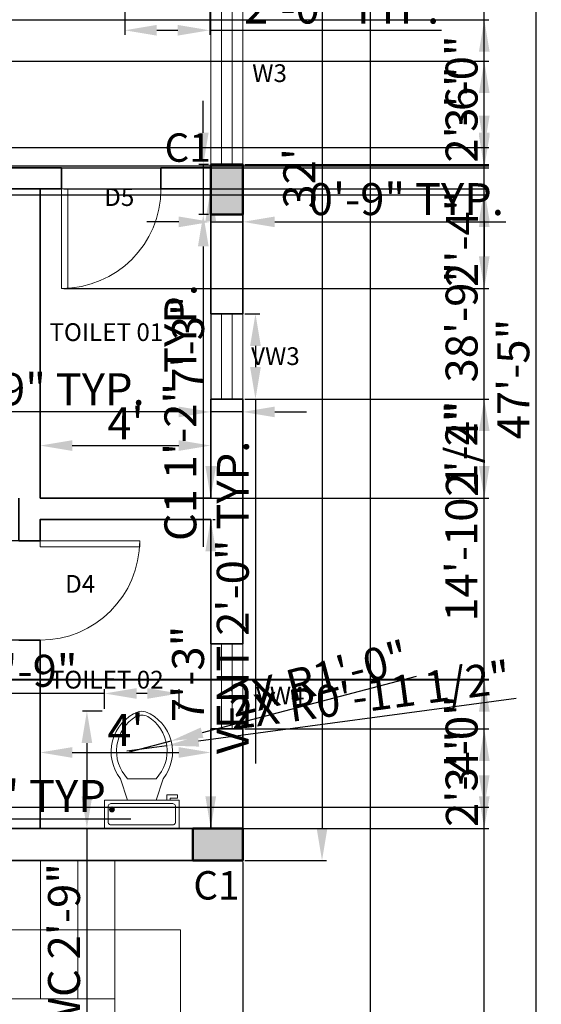
# Model space of a CAD drawing. Units: inches. Extents: x 2621 to 6190, y 513 to 1320.
# Tile 9 of 11: x 3160 to 3306, y 661 to 939. Entities that reach past the tile are written whole.
import ezdxf

# ---------------------------------------------------------------- set-up
doc = ezdxf.new("R2010")
doc.units = ezdxf.units.IN
for name, color, linetype, lineweight in [('A-ANNO-DIMS', 5, 'Continuous', 18), ('A-ANNO-TEXT', 7, 'Continuous', 18), ('A-AREA-IDEN', 7, 'Continuous', 25), ('A-FLOR-CASE', 30, 'Continuous', 18), ('A-FLOR-FIXT', 30, 'Continuous', 18), ('A-WALL', 7, 'Continuous', 35), ('C-PROP', 7, 'Continuous', 25), ('columns', 2, 'Continuous', 50), ('door', 1, 'Continuous', 18), ('S-COLS-IDEN', 2, 'Continuous', 25), ('S-COLS-PATT', 2, 'Continuous', 13), ('stairs', 104, 'Continuous', 18), ('window', 172, 'Continuous', 18)]:
    doc.layers.add(name, color=color, linetype=linetype, lineweight=lineweight)
doc.styles.get("Standard").update_dxf_attribs({"font": 'arial.ttf'})
doc.dimstyles.new('ISO-25', dxfattribs={"dimtxt": 9, "dimasz": 9, "dimexe": 1.25, "dimexo": 0.625, "dimtad": 1, "dimlunit": 3, "dimtxsty": 'Standard', "dimcen": 2.5, "dimadec": 0, "dimazin": 0, "dimtfac": 1, "dimtmove": 0, "dimatfit": 3, "dimfxl": 1, "dimarcsym": 0})

# ---------------------------------------------------------------- blocks, each defined once
blk = doc.blocks.new('*U4')
for p, q in [((0, 0), (0, 6)), ((28, 0), (28, 6))]:
    blk.add_line(p, q)
blk.add_lwpolyline([(0, 0), (0, -28), (1.75, -28), (1.75, 0)], close=True)
blk.add_arc((0, 0), 28, 270, 0)
blk = doc.blocks.new('*U3')
for p, q in [((-28, 0), (-28, 6)), ((0, 0), (0, 6))]:
    blk.add_line(p, q)
blk.add_lwpolyline([(0, 0), (0, -28), (-1.75, -28), (-1.75, 0)], close=True)
blk.add_arc((0, 0), 28, 180, 270)
blk = doc.blocks.new('Toilet - top')
for p, q in [((9.5, -6), (9.5, -2)), ((-8, -8.5), (-8, -8)), ((-7, -8), (-7, -9.5)), ((-4, -8), (-6, -14)), ((4, -8), (6, -14)), ((-10, -8.5), (-8, -8.5)), ((-10, -9.5), (-10, -8.5)), ((-7, -9.5), (-10, -9.5)), ((4, -14), (-4, -14))]:
    blk.add_line(p, q)
blk.add_lwpolyline([(10.5, -8), (10.5, 0), (-10.5, 0), (-10.5, -8)], close=True)
for points in [[(-9.5, -2), (-9.5, -6)], [(8.5, -1), (-8.5, -1)], [(-8.5, -7), (8.5, -7)]]:
    blk.add_lwpolyline(points)
for centre, radius, start, end in [((-8.62, -1.88), 0.884, 81.8699, 188.1301), ((8.62, -1.88), 0.884, 351.8699, 98.1301), ((-8.62, -6.12), 0.884, 171.8699, 278.1301), ((8.62, -6.12), 0.884, 261.8699, 8.1301), ((3.52, -21.58), 12.17, 141.4691, 247.9714), ((4.2, -21.82), 11.33, 136.3677, 238.9468), ((-3.52, -21.58), 12.17, 292.0284, 38.5307), ((-4.2, -21.82), 11.33, 301.053, 43.6321), ((0, -27.88), 4, 245.7318, 294.2682), ((0, -29), 4, 254.8605, 285.1395)]:
    blk.add_arc(centre, radius, start, end)
blk = doc.blocks.new('*D29')
at = {"layer": 'A-ANNO-DIMS', "color": 0, "lineweight": -2, "transparency": 16777216}
for p, q in [((3214.01, 797.89), (3214.63, 797.89)), ((3213.38, 788.89), (3213.38, 719.89)), ((3214.01, 710.89), (3214.63, 710.89))]:
    blk.add_line(p, q, dxfattribs=at)
at = {"layer": 'A-ANNO-DIMS', "color": 0, "transparency": 16777216}
for points in [[(3211.88, 788.89), (3214.88, 788.89), (3213.38, 797.89)], [(3211.88, 719.89), (3214.88, 719.89), (3213.38, 710.89)]]:
    blk.add_solid(points, dxfattribs=at)
at = {"layer": 'Defpoints', "color": 0, "transparency": 16777216}
for p in [(3213.38, 797.89), (3213.38, 710.89), (3213.38, 710.89)]:
    blk.add_point(p, dxfattribs=at)
at = {"layer": 'A-ANNO-DIMS', "color": 0, "transparency": 16777216, "insert": (3208.16, 754.39), "char_height": 9, "attachment_point": 5, "rotation": 90}
blk.add_mtext('7\'-3"', dxfattribs=at)
blk = doc.blocks.new('*D30')
at = {"layer": 'A-ANNO-DIMS', "color": 0, "lineweight": -2, "transparency": 16777216}
for p, q in [((3165.38, 729.52), (3165.38, 733.53)), ((3174.38, 732.28), (3204.38, 732.28)), ((3213.38, 731.63), (3213.38, 733.53))]:
    blk.add_line(p, q, dxfattribs=at)
at = {"layer": 'A-ANNO-DIMS', "color": 0, "transparency": 16777216}
for points in [[(3174.38, 733.78), (3174.38, 730.78), (3165.38, 732.28)], [(3204.38, 733.78), (3204.38, 730.78), (3213.38, 732.28)]]:
    blk.add_solid(points, dxfattribs=at)
at = {"layer": 'Defpoints', "color": 0, "transparency": 16777216}
for p in [(3213.38, 732.28), (3213.38, 731.01), (3165.38, 728.89)]:
    blk.add_point(p, dxfattribs=at)
at = {"layer": 'A-ANNO-DIMS', "color": 0, "transparency": 16777216, "insert": (3189.38, 737.4), "char_height": 9, "attachment_point": 5}
blk.add_mtext("4'", dxfattribs=at)
blk = doc.blocks.new('*D31')
at = {"layer": 'A-ANNO-DIMS', "color": 0, "lineweight": -2, "transparency": 16777216}
for p, q in [((3165.38, 819.75), (3165.38, 817.42)), ((3174.38, 818.67), (3204.38, 818.67)), ((3213.38, 819.75), (3213.38, 817.42))]:
    blk.add_line(p, q, dxfattribs=at)
at = {"layer": 'A-ANNO-DIMS', "color": 0, "transparency": 16777216}
for points in [[(3174.38, 820.17), (3174.38, 817.17), (3165.38, 818.67)], [(3204.38, 820.17), (3204.38, 817.17), (3213.38, 818.67)]]:
    blk.add_solid(points, dxfattribs=at)
at = {"layer": 'Defpoints', "color": 0, "transparency": 16777216}
for p in [(3165.38, 820.37), (3213.38, 820.37), (3213.38, 818.67)]:
    blk.add_point(p, dxfattribs=at)
at = {"layer": 'A-ANNO-DIMS', "color": 0, "transparency": 16777216, "insert": (3189.38, 823.79), "char_height": 9, "attachment_point": 5}
blk.add_mtext("4'", dxfattribs=at)
blk = doc.blocks.new('*D32')
at = {"layer": 'A-ANNO-DIMS', "color": 0, "lineweight": -2, "transparency": 16777216}
for p, q in [((3207.01, 890.89), (3214.63, 890.89)), ((3213.38, 881.89), (3213.38, 812.89)), ((3207.01, 803.89), (3214.63, 803.89))]:
    blk.add_line(p, q, dxfattribs=at)
at = {"layer": 'A-ANNO-DIMS', "color": 0, "transparency": 16777216}
for points in [[(3211.88, 881.89), (3214.88, 881.89), (3213.38, 890.89)], [(3211.88, 812.89), (3214.88, 812.89), (3213.38, 803.89)]]:
    blk.add_solid(points, dxfattribs=at)
at = {"layer": 'Defpoints', "color": 0, "transparency": 16777216}
for p in [(3206.38, 890.89), (3206.38, 803.89), (3213.38, 803.89)]:
    blk.add_point(p, dxfattribs=at)
at = {"layer": 'A-ANNO-DIMS', "color": 0, "transparency": 16777216, "insert": (3208.16, 847.39), "char_height": 9, "attachment_point": 5, "rotation": 90}
blk.add_mtext('7\'-3"', dxfattribs=at)
blk = doc.blocks.new('*D35')
at = {"layer": 'A-ANNO-DIMS', "color": 0, "lineweight": -2, "transparency": 16777216}
for p, q in [((3223.01, 1085.89), (3245.96, 1085.89)), ((3244.71, 1076.89), (3244.71, 710.89)), ((3223.01, 701.89), (3245.96, 701.89))]:
    blk.add_line(p, q, dxfattribs=at)
at = {"layer": 'A-ANNO-DIMS', "color": 0, "transparency": 16777216}
for points in [[(3243.21, 1076.89), (3246.21, 1076.89), (3244.71, 1085.89)], [(3243.21, 710.89), (3246.21, 710.89), (3244.71, 701.89)]]:
    blk.add_solid(points, dxfattribs=at)
at = {"layer": 'Defpoints', "color": 0, "transparency": 16777216}
for p in [(3222.38, 1085.89), (3222.38, 701.89), (3244.71, 701.89)]:
    blk.add_point(p, dxfattribs=at)
at = {"layer": 'A-ANNO-DIMS', "color": 0, "transparency": 16777216, "insert": (3239.48, 893.89), "char_height": 9, "attachment_point": 5, "rotation": 90}
blk.add_mtext("32'", dxfattribs=at)
blk = doc.blocks.new('*D39')
at = {"layer": 'A-ANNO-DIMS', "color": 0, "lineweight": -2, "transparency": 16777216}
for p, q in [((3259.01, 1121.89), (3306.19, 1121.89)), ((3304.94, 1112.89), (3304.94, 561.89)), ((3259.01, 552.89), (3306.19, 552.89))]:
    blk.add_line(p, q, dxfattribs=at)
at = {"layer": 'A-ANNO-DIMS', "color": 0, "transparency": 16777216}
for points in [[(3303.44, 1112.89), (3306.44, 1112.89), (3304.94, 1121.89)], [(3303.44, 561.89), (3306.44, 561.89), (3304.94, 552.89)]]:
    blk.add_solid(points, dxfattribs=at)
at = {"layer": 'Defpoints', "color": 0, "transparency": 16777216}
for p in [(3258.38, 1121.89), (3258.38, 552.89), (3304.94, 552.89)]:
    blk.add_point(p, dxfattribs=at)
at = {"layer": 'A-ANNO-DIMS', "color": 0, "transparency": 16777216, "insert": (3299.73, 837.39), "char_height": 9, "attachment_point": 5, "rotation": 90}
blk.add_mtext('47\'-5"', dxfattribs=at)
blk = doc.blocks.new('WIN-VENT-24IN')
for p, q in [((9, 24), (0, 24)), ((0, 24), (0, 0)), ((3, 24), (3, 0)), ((6, 24), (6, 0)), ((9, 0), (9, 24)), ((0, 0), (9, 0))]:
    blk.add_line(p, q)
blk = doc.blocks.new('WIN-48IN')
for p, q in [((48, 9), (0, 9)), ((0, 9), (0, 0)), ((48, 0), (48, 9)), ((0, 6), (48, 6)), ((0, 3), (48, 3)), ((0, 0), (48, 0))]:
    blk.add_line(p, q)
blk = doc.blocks.new('COL-C1-9X14')
blk.add_lwpolyline([(0, 0), (0, 9), (14, 9), (14, 0)], close=True)
blk = doc.blocks.new('*D51')
at = {"layer": 'A-ANNO-DIMS', "color": 0, "lineweight": -2, "transparency": 16777216}
for p, q in [((3211.28, 906.74), (3211.28, 915.74)), ((3212.76, 897.74), (3210.03, 897.74)), ((3211.28, 897.74), (3211.28, 883.74)), ((3212.76, 883.74), (3210.03, 883.74)), ((3211.28, 874.74), (3211.28, 790.17))]:
    blk.add_line(p, q, dxfattribs=at)
at = {"layer": 'A-ANNO-DIMS', "color": 0, "transparency": 16777216}
for points in [[(3209.78, 906.74), (3212.78, 906.74), (3211.28, 897.74)], [(3209.78, 874.74), (3212.78, 874.74), (3211.28, 883.74)]]:
    blk.add_solid(points, dxfattribs=at)
at = {"layer": 'Defpoints', "color": 0, "transparency": 16777216}
for p in [(3213.38, 897.74), (3211.28, 883.74), (3213.38, 883.74)]:
    blk.add_point(p, dxfattribs=at)
at = {"layer": 'A-ANNO-DIMS', "color": 0, "transparency": 16777216, "insert": (3206, 827.96), "char_height": 9, "attachment_point": 5, "rotation": 90}
blk.add_mtext('C1 1\'-2" TYP.', dxfattribs=at)
blk = doc.blocks.new('*D52')
at = {"layer": 'A-ANNO-DIMS', "color": 0, "lineweight": -2, "transparency": 16777216}
for p, q in [((3204.38, 881.64), (3195.38, 881.64)), ((3213.38, 883.12), (3213.38, 880.39)), ((3213.38, 881.64), (3222.38, 881.64)), ((3222.38, 883.12), (3222.38, 880.39)), ((3231.38, 881.64), (3296.49, 881.64))]:
    blk.add_line(p, q, dxfattribs=at)
at = {"layer": 'A-ANNO-DIMS', "color": 0, "transparency": 16777216}
for points in [[(3204.38, 883.14), (3204.38, 880.14), (3213.38, 881.64)], [(3231.38, 883.14), (3231.38, 880.14), (3222.38, 881.64)]]:
    blk.add_solid(points, dxfattribs=at)
at = {"layer": 'Defpoints', "color": 0, "transparency": 16777216}
for p in [(3213.38, 883.74), (3222.38, 883.74), (3222.38, 881.64)]:
    blk.add_point(p, dxfattribs=at)
at = {"layer": 'A-ANNO-DIMS', "color": 0, "transparency": 16777216, "insert": (3268.44, 886.87), "char_height": 9, "attachment_point": 5}
blk.add_mtext('0\'-9" TYP.', dxfattribs=at)
blk = doc.blocks.new('*D53')
at = {"layer": 'A-ANNO-DIMS', "color": 0, "lineweight": -2, "transparency": 16777216}
for p, q in [((3012.32, 713.59), (3003.32, 713.59)), ((3021.32, 711.51), (3021.32, 714.84)), ((3021.32, 713.59), (3039.32, 713.59)), ((3039.32, 711.51), (3039.32, 714.84)), ((3048.32, 713.59), (3190.87, 713.59))]:
    blk.add_line(p, q, dxfattribs=at)
at = {"layer": 'A-ANNO-DIMS', "color": 0, "transparency": 16777216}
for points in [[(3012.32, 715.09), (3012.32, 712.09), (3021.32, 713.59)], [(3048.32, 715.09), (3048.32, 712.09), (3039.32, 713.59)]]:
    blk.add_solid(points, dxfattribs=at)
at = {"layer": 'Defpoints', "color": 0, "transparency": 16777216}
for p in [(3039.32, 713.59), (3021.32, 710.89), (3039.32, 710.89)]:
    blk.add_point(p, dxfattribs=at)
at = {"layer": 'A-ANNO-DIMS', "color": 0, "transparency": 16777216, "insert": (3124.09, 718.87), "char_height": 9, "attachment_point": 5}
blk.add_mtext('C2 COLUMN 1\'-6" TYP.', dxfattribs=at)
blk = doc.blocks.new('*D57')
at = {"layer": 'A-ANNO-DIMS', "color": 0, "lineweight": -2, "transparency": 16777216}
for p, q in [((3223.01, 855.74), (3227.23, 855.74)), ((3225.98, 846.74), (3225.98, 840.74)), ((3223.01, 831.74), (3227.23, 831.74)), ((3225.98, 831.74), (3225.98, 729.14))]:
    blk.add_line(p, q, dxfattribs=at)
at = {"layer": 'A-ANNO-DIMS', "color": 0, "transparency": 16777216}
for points in [[(3224.48, 846.74), (3227.48, 846.74), (3225.98, 855.74)], [(3224.48, 840.74), (3227.48, 840.74), (3225.98, 831.74)]]:
    blk.add_solid(points, dxfattribs=at)
at = {"layer": 'Defpoints', "color": 0, "transparency": 16777216}
for p in [(3222.38, 855.74), (3222.38, 831.74), (3225.98, 831.74)]:
    blk.add_point(p, dxfattribs=at)
at = {"layer": 'A-ANNO-DIMS', "color": 0, "transparency": 16777216, "insert": (3220.76, 775.94), "char_height": 9, "attachment_point": 5, "rotation": 90}
blk.add_mtext('VENT 2\'-0" TYP.', dxfattribs=at)
blk = doc.blocks.new('*D58')
at = {"layer": 'A-ANNO-DIMS', "color": 0, "lineweight": -2, "transparency": 16777216}
for p, q in [((3213.38, 831.12), (3213.38, 826.89)), ((3222.38, 831.12), (3222.38, 826.89)), ((3204.38, 828.14), (3139.27, 828.14)), ((3222.38, 828.14), (3213.38, 828.14)), ((3231.38, 828.14), (3240.38, 828.14))]:
    blk.add_line(p, q, dxfattribs=at)
at = {"layer": 'A-ANNO-DIMS', "color": 0, "transparency": 16777216}
for points in [[(3204.38, 829.64), (3204.38, 826.64), (3213.38, 828.14)], [(3231.38, 829.64), (3231.38, 826.64), (3222.38, 828.14)]]:
    blk.add_solid(points, dxfattribs=at)
at = {"layer": 'Defpoints', "color": 0, "transparency": 16777216}
for p in [(3213.38, 831.74), (3222.38, 831.74), (3213.38, 828.14)]:
    blk.add_point(p, dxfattribs=at)
at = {"layer": 'A-ANNO-DIMS', "color": 0, "transparency": 16777216, "insert": (3167.33, 833.37), "char_height": 9, "attachment_point": 5}
blk.add_mtext('0\'-9" TYP.', dxfattribs=at)
blk = doc.blocks.new('*D62')
at = {"layer": 'A-ANNO-DIMS', "color": 0, "lineweight": -2, "transparency": 16777216}
for p, q in [((3189.19, 945.12), (3189.19, 934.32)), ((3213.1, 945.12), (3213.1, 934.32)), ((3198.19, 935.57), (3204.1, 935.57)), ((3213.1, 935.57), (3278.36, 935.57))]:
    blk.add_line(p, q, dxfattribs=at)
at = {"layer": 'A-ANNO-DIMS', "color": 0, "transparency": 16777216}
for points in [[(3198.19, 937.07), (3198.19, 934.07), (3189.19, 935.57)], [(3204.1, 937.07), (3204.1, 934.07), (3213.1, 935.57)]]:
    blk.add_solid(points, dxfattribs=at)
at = {"layer": 'Defpoints', "color": 0, "transparency": 16777216}
for p in [(3189.19, 945.74), (3213.1, 945.74), (3213.1, 935.57)]:
    blk.add_point(p, dxfattribs=at)
at = {"layer": 'A-ANNO-DIMS', "color": 0, "transparency": 16777216, "insert": (3250.23, 940.79), "char_height": 9, "attachment_point": 5}
blk.add_mtext('2\'-0" TYP.', dxfattribs=at)
blk = doc.blocks.new('*D71')
at = {"layer": 'A-ANNO-DIMS', "color": 0, "lineweight": -2, "transparency": 16777216}
for p, q in [((3182.86, 743.94), (3177.28, 743.94)), ((3178.53, 734.94), (3178.53, 719.89)), ((3182.86, 710.89), (3177.28, 710.89)), ((3178.53, 710.89), (3178.53, 651.91))]:
    blk.add_line(p, q, dxfattribs=at)
at = {"layer": 'A-ANNO-DIMS', "color": 0, "transparency": 16777216}
for points in [[(3177.03, 734.94), (3180.03, 734.94), (3178.53, 743.94)], [(3177.03, 719.89), (3180.03, 719.89), (3178.53, 710.89)]]:
    blk.add_solid(points, dxfattribs=at)
at = {"layer": 'Defpoints', "color": 0, "transparency": 16777216}
for p in [(3183.49, 743.94), (3178.53, 710.89), (3183.49, 710.89)]:
    blk.add_point(p, dxfattribs=at)
at = {"layer": 'A-ANNO-DIMS', "color": 0, "transparency": 16777216, "insert": (3173.25, 676.9), "char_height": 9, "attachment_point": 5, "rotation": 90}
blk.add_mtext('WC 2\'-9"', dxfattribs=at)
blk = doc.blocks.new('*D72')
at = {"layer": 'A-ANNO-DIMS', "color": 0, "lineweight": -2, "transparency": 16777216}
for p, q in [((3183.49, 748.89), (3150.16, 748.89)), ((3183.49, 744.56), (3183.49, 750.14)), ((3195.49, 748.89), (3192.49, 748.89)), ((3204.49, 744.56), (3204.49, 750.14))]:
    blk.add_line(p, q, dxfattribs=at)
at = {"layer": 'A-ANNO-DIMS', "color": 0, "transparency": 16777216}
for points in [[(3192.49, 750.39), (3192.49, 747.39), (3183.49, 748.89)], [(3195.49, 750.39), (3195.49, 747.39), (3204.49, 748.89)]]:
    blk.add_solid(points, dxfattribs=at)
at = {"layer": 'Defpoints', "color": 0, "transparency": 16777216}
for p in [(3183.49, 748.89), (3183.49, 743.94), (3204.49, 743.94)]:
    blk.add_point(p, dxfattribs=at)
at = {"layer": 'A-ANNO-DIMS', "color": 0, "transparency": 16777216, "insert": (3162.32, 754.11), "char_height": 9, "attachment_point": 5}
blk.add_mtext('1\'-9"', dxfattribs=at)
blk = doc.blocks.new('*D82')
at = {"layer": 'A-ANNO-DIMS', "color": 0, "lineweight": -2, "transparency": 16777216}
for p, q in [((2924.85, 889.24), (3291.63, 889.24)), ((3290.38, 719.89), (3290.38, 880.24)), ((2917.49, 710.89), (3291.63, 710.89))]:
    blk.add_line(p, q, dxfattribs=at)
at = {"layer": 'A-ANNO-DIMS', "color": 0, "transparency": 16777216}
for points in [[(3288.88, 880.24), (3291.88, 880.24), (3290.38, 889.24)], [(3288.88, 719.89), (3291.88, 719.89), (3290.38, 710.89)]]:
    blk.add_solid(points, dxfattribs=at)
at = {"layer": 'Defpoints', "color": 0, "transparency": 16777216}
for p in [(2924.22, 889.24), (3290.38, 889.24), (2916.87, 710.89)]:
    blk.add_point(p, dxfattribs=at)
at = {"layer": 'A-ANNO-DIMS', "color": 0, "transparency": 16777216, "insert": (3285.1, 800.07), "char_height": 9, "attachment_point": 5, "rotation": 90}
blk.add_mtext('14\'-10 1/2"', dxfattribs=at)
blk = doc.blocks.new('*D83')
at = {"layer": 'A-ANNO-DIMS', "color": 0, "lineweight": -2, "transparency": 16777216}
for p, q in [((3028.01, 1085.89), (3291.63, 1085.89)), ((3290.38, 906.39), (3290.38, 1076.89)), ((3028.01, 897.39), (3291.63, 897.39))]:
    blk.add_line(p, q, dxfattribs=at)
at = {"layer": 'A-ANNO-DIMS', "color": 0, "transparency": 16777216}
for points in [[(3288.88, 1076.89), (3291.88, 1076.89), (3290.38, 1085.89)], [(3288.88, 906.39), (3291.88, 906.39), (3290.38, 897.39)]]:
    blk.add_solid(points, dxfattribs=at)
at = {"layer": 'Defpoints', "color": 0, "transparency": 16777216}
for p in [(3027.38, 1085.89), (3290.38, 1085.89), (3027.38, 897.39)]:
    blk.add_point(p, dxfattribs=at)
at = {"layer": 'A-ANNO-DIMS', "color": 0, "transparency": 16777216, "insert": (3285.1, 991.64), "char_height": 9, "attachment_point": 5, "rotation": 90}
blk.add_mtext('15\'-8 1/2"', dxfattribs=at)
blk = doc.blocks.new('*D84')
at = {"layer": 'A-ANNO-DIMS', "color": 0, "lineweight": -2, "transparency": 16777216}
for p, q in [((3223.01, 1085.89), (3291.63, 1085.89)), ((3290.38, 906.74), (3290.38, 1076.89)), ((3223.01, 897.74), (3291.63, 897.74))]:
    blk.add_line(p, q, dxfattribs=at)
at = {"layer": 'A-ANNO-DIMS', "color": 0, "transparency": 16777216}
for points in [[(3288.88, 1076.89), (3291.88, 1076.89), (3290.38, 1085.89)], [(3288.88, 906.74), (3291.88, 906.74), (3290.38, 897.74)]]:
    blk.add_solid(points, dxfattribs=at)
at = {"layer": 'Defpoints', "color": 0, "transparency": 16777216}
for p in [(3222.38, 1085.89), (3290.38, 1085.89), (3222.38, 897.74)]:
    blk.add_point(p, dxfattribs=at)
at = {"layer": 'A-ANNO-DIMS', "color": 0, "transparency": 16777216, "insert": (3285.16, 991.82), "char_height": 9, "attachment_point": 5, "rotation": 90}
blk.add_mtext('15\'-8"', dxfattribs=at)
blk = doc.blocks.new('*D91')
at = {"layer": 'A-ANNO-DIMS', "color": 0, "lineweight": -2, "transparency": 16777216}
for p, q in [((3223.01, 1085.89), (3291.63, 1085.89)), ((3290.38, 629.89), (3290.38, 1076.89)), ((3223.01, 620.89), (3291.63, 620.89))]:
    blk.add_line(p, q, dxfattribs=at)
at = {"layer": 'A-ANNO-DIMS', "color": 0, "transparency": 16777216}
for points in [[(3288.88, 1076.89), (3291.88, 1076.89), (3290.38, 1085.89)], [(3288.88, 629.89), (3291.88, 629.89), (3290.38, 620.89)]]:
    blk.add_solid(points, dxfattribs=at)
at = {"layer": 'Defpoints', "color": 0, "transparency": 16777216}
for p in [(3222.38, 1085.89), (3290.38, 1085.89), (3222.38, 620.89)]:
    blk.add_point(p, dxfattribs=at)
at = {"layer": 'A-ANNO-DIMS', "color": 0, "transparency": 16777216, "insert": (3285.16, 853.39), "char_height": 9, "attachment_point": 5, "rotation": 90}
blk.add_mtext('38\'-9"', dxfattribs=at)
blk = doc.blocks.new('*D92')
at = {"layer": 'A-ANNO-DIMS', "color": 0, "lineweight": -2, "transparency": 16777216}
for p, q in [((3222.38, 701.26), (3222.38, 519.64)), ((2730.38, 686.26), (2730.38, 519.64)), ((2739.38, 520.89), (3213.38, 520.89))]:
    blk.add_line(p, q, dxfattribs=at)
at = {"layer": 'A-ANNO-DIMS', "color": 0, "transparency": 16777216}
for points in [[(2739.38, 522.39), (2739.38, 519.39), (2730.38, 520.89)], [(3213.38, 522.39), (3213.38, 519.39), (3222.38, 520.89)]]:
    blk.add_solid(points, dxfattribs=at)
at = {"layer": 'Defpoints', "color": 0, "transparency": 16777216}
for p in [(3222.38, 701.89), (2730.38, 686.89), (3222.38, 520.89)]:
    blk.add_point(p, dxfattribs=at)
at = {"layer": 'A-ANNO-DIMS', "color": 0, "transparency": 16777216, "insert": (2976.38, 526.11), "char_height": 9, "attachment_point": 5}
blk.add_mtext('41\'-0"', dxfattribs=at)
blk = doc.blocks.new('*D95')
at = {"layer": 'A-ANNO-DIMS', "color": 0, "lineweight": -2, "transparency": 16777216}
for p, q in [((2788.01, 752.76), (3291.63, 752.76)), ((3290.38, 725.89), (3290.38, 743.76)), ((2788.01, 716.89), (3291.63, 716.89))]:
    blk.add_line(p, q, dxfattribs=at)
at = {"layer": 'A-ANNO-DIMS', "color": 0, "transparency": 16777216}
for points in [[(3288.88, 743.76), (3291.88, 743.76), (3290.38, 752.76)], [(3288.88, 725.89), (3291.88, 725.89), (3290.38, 716.89)]]:
    blk.add_solid(points, dxfattribs=at)
at = {"layer": 'Defpoints', "color": 0, "transparency": 16777216}
for p in [(2787.38, 752.76), (3290.38, 752.76), (2787.38, 716.89)]:
    blk.add_point(p, dxfattribs=at)
at = {"layer": 'A-ANNO-DIMS', "color": 0, "transparency": 16777216, "insert": (3285.16, 734.83), "char_height": 9, "attachment_point": 5, "rotation": 90}
blk.add_mtext('3\'-0"', dxfattribs=at)
blk = doc.blocks.new('*D96')
at = {"layer": 'A-ANNO-DIMS', "color": 0, "lineweight": -2, "transparency": 16777216}
for p, q in [((3034.01, 752.89), (3291.63, 752.89)), ((3290.38, 725.89), (3290.38, 743.89)), ((3034.01, 716.89), (3291.63, 716.89))]:
    blk.add_line(p, q, dxfattribs=at)
at = {"layer": 'A-ANNO-DIMS', "color": 0, "transparency": 16777216}
for points in [[(3288.88, 743.89), (3291.88, 743.89), (3290.38, 752.89)], [(3288.88, 725.89), (3291.88, 725.89), (3290.38, 716.89)]]:
    blk.add_solid(points, dxfattribs=at)
at = {"layer": 'Defpoints', "color": 0, "transparency": 16777216}
for p in [(3033.38, 752.89), (3290.38, 752.89), (3033.38, 716.89)]:
    blk.add_point(p, dxfattribs=at)
at = {"layer": 'A-ANNO-DIMS', "color": 0, "transparency": 16777216, "insert": (3285.16, 734.89), "char_height": 9, "attachment_point": 5, "rotation": 90}
blk.add_mtext('3\'-0"', dxfattribs=at)
blk = doc.blocks.new('*D97')
at = {"layer": 'A-ANNO-DIMS', "color": 0, "lineweight": -2, "transparency": 16777216}
for p, q in [((3164.76, 791.89), (2685.13, 791.89)), ((2686.38, 772.89), (2686.38, 782.89)), ((3164.76, 763.89), (2685.13, 763.89))]:
    blk.add_line(p, q, dxfattribs=at)
at = {"layer": 'A-ANNO-DIMS', "color": 0, "transparency": 16777216}
for points in [[(2684.88, 782.89), (2687.88, 782.89), (2686.38, 791.89)], [(2684.88, 772.89), (2687.88, 772.89), (2686.38, 763.89)]]:
    blk.add_solid(points, dxfattribs=at)
at = {"layer": 'Defpoints', "color": 0, "transparency": 16777216}
for p in [(2686.38, 791.89), (3165.38, 791.89), (3165.38, 763.89)]:
    blk.add_point(p, dxfattribs=at)
at = {"layer": 'A-ANNO-DIMS', "color": 0, "transparency": 16777216, "insert": (2681.24, 777.89), "char_height": 9, "attachment_point": 5, "rotation": 90}
blk.add_mtext('2\'-4"', dxfattribs=at)
blk = doc.blocks.new('*D98')
at = {"layer": 'A-ANNO-DIMS', "color": 0, "lineweight": -2, "transparency": 16777216}
for p, q in [((3172.01, 890.89), (3291.63, 890.89)), ((3290.38, 881.89), (3290.38, 871.89)), ((3172.01, 862.89), (3291.63, 862.89))]:
    blk.add_line(p, q, dxfattribs=at)
at = {"layer": 'A-ANNO-DIMS', "color": 0, "transparency": 16777216}
for points in [[(3288.88, 881.89), (3291.88, 881.89), (3290.38, 890.89)], [(3288.88, 871.89), (3291.88, 871.89), (3290.38, 862.89)]]:
    blk.add_solid(points, dxfattribs=at)
at = {"layer": 'Defpoints', "color": 0, "transparency": 16777216}
for p in [(3171.38, 890.89), (3171.38, 862.89), (3290.38, 862.89)]:
    blk.add_point(p, dxfattribs=at)
at = {"layer": 'A-ANNO-DIMS', "color": 0, "transparency": 16777216, "insert": (3285.24, 876.89), "char_height": 9, "attachment_point": 5, "rotation": 90}
blk.add_mtext('2\'-4"', dxfattribs=at)
blk = doc.blocks.new('*D99')
at = {"layer": 'A-ANNO-DIMS', "color": 0, "lineweight": -2, "transparency": 16777216}
for p, q in [((3034.01, 938.55), (3291.63, 938.55)), ((3290.38, 911.55), (3290.38, 929.55)), ((3034.01, 902.55), (3291.63, 902.55))]:
    blk.add_line(p, q, dxfattribs=at)
at = {"layer": 'A-ANNO-DIMS', "color": 0, "transparency": 16777216}
for points in [[(3288.88, 929.55), (3291.88, 929.55), (3290.38, 938.55)], [(3288.88, 911.55), (3291.88, 911.55), (3290.38, 902.55)]]:
    blk.add_solid(points, dxfattribs=at)
at = {"layer": 'Defpoints', "color": 0, "transparency": 16777216}
for p in [(3033.38, 938.55), (3290.38, 938.55), (3033.38, 902.55)]:
    blk.add_point(p, dxfattribs=at)
at = {"layer": 'A-ANNO-DIMS', "color": 0, "transparency": 16777216, "insert": (3285.16, 920.55), "char_height": 9, "attachment_point": 5, "rotation": 90}
blk.add_mtext('3\'-0"', dxfattribs=at)
blk = doc.blocks.new('*D100')
at = {"layer": 'A-ANNO-DIMS', "color": 0, "lineweight": -2, "transparency": 16777216}
for p, q in [((2854.01, 926.89), (3291.63, 926.89)), ((3290.38, 905.89), (3290.38, 917.89)), ((2854.01, 896.89), (3291.63, 896.89))]:
    blk.add_line(p, q, dxfattribs=at)
at = {"layer": 'A-ANNO-DIMS', "color": 0, "transparency": 16777216}
for points in [[(3288.88, 917.89), (3291.88, 917.89), (3290.38, 926.89)], [(3288.88, 905.89), (3291.88, 905.89), (3290.38, 896.89)]]:
    blk.add_solid(points, dxfattribs=at)
at = {"layer": 'Defpoints', "color": 0, "transparency": 16777216}
for p in [(2853.38, 926.89), (3290.38, 926.89), (2853.38, 896.89)]:
    blk.add_point(p, dxfattribs=at)
at = {"layer": 'A-ANNO-DIMS', "color": 0, "transparency": 16777216, "insert": (3285.16, 911.89), "char_height": 9, "attachment_point": 5, "rotation": 90}
blk.add_mtext('2\'-6"', dxfattribs=at)
blk = doc.blocks.new('*D111')
at = {"layer": 'A-ANNO-DIMS', "color": 0, "lineweight": -2, "transparency": 16777216}
for p, q in [((3223.01, 738.89), (3291.63, 738.89)), ((3290.38, 719.89), (3290.38, 729.89)), ((3214.01, 710.89), (3291.63, 710.89))]:
    blk.add_line(p, q, dxfattribs=at)
at = {"layer": 'A-ANNO-DIMS', "color": 0, "transparency": 16777216}
for points in [[(3288.88, 729.89), (3291.88, 729.89), (3290.38, 738.89)], [(3288.88, 719.89), (3291.88, 719.89), (3290.38, 710.89)]]:
    blk.add_solid(points, dxfattribs=at)
at = {"layer": 'Defpoints', "color": 0, "transparency": 16777216}
for p in [(3222.38, 738.89), (3290.38, 738.89), (3213.38, 710.89)]:
    blk.add_point(p, dxfattribs=at)
at = {"layer": 'A-ANNO-DIMS', "color": 0, "transparency": 16777216, "insert": (3285.24, 724.89), "char_height": 9, "attachment_point": 5, "rotation": 90}
blk.add_mtext('2\'-4"', dxfattribs=at)
blk = doc.blocks.new('*D112')
at = {"layer": 'A-ANNO-DIMS', "color": 0, "lineweight": -2, "transparency": 16777216}
for p, q in [((3223.01, 831.74), (3291.63, 831.74)), ((3290.38, 812.89), (3290.38, 822.74)), ((3214.01, 803.89), (3291.63, 803.89))]:
    blk.add_line(p, q, dxfattribs=at)
at = {"layer": 'A-ANNO-DIMS', "color": 0, "transparency": 16777216}
for points in [[(3288.88, 822.74), (3291.88, 822.74), (3290.38, 831.74)], [(3288.88, 812.89), (3291.88, 812.89), (3290.38, 803.89)]]:
    blk.add_solid(points, dxfattribs=at)
at = {"layer": 'Defpoints', "color": 0, "transparency": 16777216}
for p in [(3222.38, 831.74), (3290.38, 831.74), (3213.38, 803.89)]:
    blk.add_point(p, dxfattribs=at)
at = {"layer": 'A-ANNO-DIMS', "color": 0, "transparency": 16777216, "insert": (3285.24, 817.82), "char_height": 9, "attachment_point": 5, "rotation": 90}
blk.add_mtext('2\'-4"', dxfattribs=at)
blk = doc.blocks.new('*D115')
at = {"layer": 'A-ANNO-DIMS', "color": 0, "lineweight": -2, "transparency": 16777216}
for p, q in [((3271.18, 753.67), (3210.94, 737.85)), ((3190.47, 732.47), (3202.24, 735.56))]:
    blk.add_line(p, q, dxfattribs=at)
at = {"layer": 'A-ANNO-DIMS', "color": 0, "transparency": 16777216}
blk.add_solid([(3210.56, 739.3), (3211.32, 736.4), (3202.24, 735.56)], dxfattribs=at)
at = {"layer": 'Defpoints', "color": 0, "transparency": 16777216}
for p in [(3202.24, 735.56), (3190.47, 732.47)]:
    blk.add_point(p, dxfattribs=at)
at = {"layer": 'A-ANNO-DIMS', "color": 0, "transparency": 16777216, "insert": (3244.09, 751.95), "char_height": 9, "attachment_point": 5, "rotation": 14.7193}
blk.add_mtext('2X R1\'-0"', dxfattribs=at)
blk = doc.blocks.new('*D116')
at = {"layer": 'A-ANNO-DIMS', "color": 0, "lineweight": -2, "transparency": 16777216}
for p, q in [((3299.37, 747.44), (3209.94, 735.42)), ((3189.79, 732.71), (3201.02, 734.22))]:
    blk.add_line(p, q, dxfattribs=at)
at = {"layer": 'A-ANNO-DIMS', "color": 0, "transparency": 16777216}
blk.add_solid([(3209.74, 736.9), (3210.14, 733.93), (3201.02, 734.22)], dxfattribs=at)
at = {"layer": 'Defpoints', "color": 0, "transparency": 16777216}
for p in [(3189.79, 732.71), (3201.02, 734.22)]:
    blk.add_point(p, dxfattribs=at)
at = {"layer": 'A-ANNO-DIMS', "color": 0, "transparency": 16777216, "insert": (3258.41, 747.26), "char_height": 9, "attachment_point": 5, "rotation": 7.6596}
blk.add_mtext('2X R0\'-11 1/2"', dxfattribs=at)

msp = doc.modelspace()

# ---------------------------------------------------------------- hatches: boundary and pattern name
at = {"layer": 'S-COLS-PATT'}
h = msp.add_hatch(color=256, dxfattribs=at)
h.dxf.hatch_style = 1
h.paths.add_polyline_path([(2787.381, 1085.89), (2778.381, 1085.89), (2778.381, 1071.89), (2787.381, 1071.89)])
h.paths.add_polyline_path([(3222.381, 1085.89), (3208.381, 1085.89), (3208.381, 1076.89), (3222.381, 1076.89)])
h.paths.add_polyline_path([(3041.381, 1085.89), (3027.381, 1085.89), (3027.381, 1076.89), (3041.381, 1076.89)])
h.paths.add_polyline_path([(2916.381, 1085.89), (2907.381, 1085.89), (2907.381, 1076.89), (2916.381, 1076.89)])
h.paths.add_polyline_path([(2916.381, 1076.89), (2913.381, 1076.89), (2913.381, 1071.89), (2916.381, 1071.89)])
h.paths.add_polyline_path([(2913.381, 1076.89), (2907.381, 1076.89), (2907.381, 1071.89), (2913.381, 1071.89)])
h.paths.add_polyline_path([(2787.381, 896.89), (2778.381, 896.89), (2778.381, 882.89), (2787.381, 882.89)])
h.paths.add_polyline_path([(2924.221, 898.241), (2910.221, 898.241), (2910.221, 889.241), (2924.221, 889.241)])
h.paths.add_polyline_path([(3036.381, 896.89), (3033.381, 896.89), (3027.381, 897.385), (3027.381, 883.385), (3033.381, 883.385), (3033.381, 890.89), (3036.381, 890.89)])
h.paths.add_polyline_path([(3036.381, 890.89), (3033.381, 890.89), (3033.381, 883.385), (3036.381, 883.385)], flags=17)
h.paths.add_polyline_path([(3222.381, 897.745), (3213.381, 897.745), (3213.381, 883.745), (3222.381, 883.745)])
h.paths.add_polyline_path([(3222.381, 710.89), (3208.381, 710.89), (3208.381, 701.89), (3222.381, 701.89)])
h.paths.add_polyline_path([(3039.318, 710.89), (3021.318, 710.89), (3021.318, 701.89), (3039.318, 701.89)])
h.paths.add_polyline_path([(2796.381, 710.89), (2778.381, 710.89), (2778.381, 701.89), (2796.381, 701.89)])

# ---------------------------------------------------------------- linework, layer by layer
at = {"layer": 'A-FLOR-CASE'}
msp.add_lwpolyline([(3165.381, 869.2), (3165.263, 869.2)], dxfattribs=at)
at = {"layer": 'A-WALL'}
for p, q in [((3171.381, 896.89), (3036.381, 896.89)), ((3171.381, 890.89), (3171.381, 896.89)), ((3213.381, 896.89), (3199.381, 896.89)), ((3199.381, 890.89), (3199.381, 896.89)), ((3213.381, 897.745), (3222.381, 897.745)), ((3213.381, 855.745), (3213.381, 897.745)), ((3222.381, 855.745), (3222.381, 897.745)), ((3171.381, 890.89), (3036.381, 890.89)), ((3165.381, 803.89), (3165.381, 890.89)), ((3213.381, 890.89), (3199.381, 890.89)), ((3213.381, 855.745), (3222.381, 855.745)), ((3213.381, 803.89), (3213.381, 831.745)), ((3213.381, 831.745), (3222.381, 831.745)), ((3222.381, 762.89), (3222.381, 831.745)), ((3213.381, 762.89), (3213.381, 797.89)), ((3159.381, 763.89), (3165.381, 763.89)), ((3165.381, 710.89), (3165.381, 763.89)), ((3222.381, 762.89), (3213.381, 762.89)), ((3213.381, 710.89), (3213.381, 738.89)), ((3222.381, 738.89), (3213.381, 738.89)), ((3222.381, 701.89), (3222.381, 738.89)), ((3125.887, 710.89), (3213.381, 710.89)), ((3125.887, 701.89), (3222.381, 701.89))]:
    msp.add_line(p, q, dxfattribs=at)
for points in [[(3213.381, 797.89), (3199.381, 797.89), (3165.381, 797.89), (3165.381, 791.89), (3159.381, 791.89), (3159.381, 803.89)], [(3165.381, 803.89), (3199.381, 803.89), (3213.381, 803.89)]]:
    msp.add_lwpolyline(points, dxfattribs=at)
at = {"layer": 'C-PROP'}
msp.add_lwpolyline([(3258.381, 552.89), (3258.381, 1121.89), (2742.381, 1121.89), (2718.381, 552.89)], close=True, dxfattribs=at)
at = {"layer": 'columns'}
msp.add_lwpolyline([(3208.381, 701.89), (3208.381, 710.89), (3222.381, 710.89), (3222.381, 701.89)], close=True, dxfattribs=at)
at = {"layer": 'stairs'}
for p, q in [((3165.485, 701.89), (3165.485, 662.89)), ((3175.933, 701.89), (3175.933, 662.89)), ((3186.381, 701.89), (3186.381, 620.89)), ((3186.381, 701.89), (3186.381, 662.89)), ((3222.381, 701.89), (3222.381, 620.89)), ((3204.871, 682.39), (3138.49, 682.39)), ((3204.871, 640.39), (3204.871, 682.39)), ((3186.381, 662.89), (3104.102, 662.89))]:
    msp.add_line(p, q, dxfattribs=at)

# ---------------------------------------------------------------- block references
at = {"layer": 'A-FLOR-FIXT', "rotation": 180}
msp.add_blockref('Toilet - top', (3193.988, 710.89), dxfattribs=at)
at = {"layer": 'columns', "rotation": 269.9999999999969}
msp.add_blockref('COL-C1-9X14', (3213.381, 897.745), dxfattribs=at)
at = {"layer": 'door'}
msp.add_blockref('*U4', (3171.381, 890.89), dxfattribs=at)
at = {"layer": 'door', "rotation": 90}
msp.add_blockref('*U3', (3165.381, 791.89), dxfattribs=at)
at = {"layer": 'window'}
for name, p, rotation in [('WIN-48IN', (3222.381, 897.745), 89.99999999999805), ('WIN-VENT-24IN', (3222.381, 855.745), 180), ('WIN-VENT-24IN', (3222.381, 762.89), 180)]:
    msp.add_blockref(name, p, dxfattribs=dict(at, rotation=rotation))

# ---------------------------------------------------------------- texts
at = {"layer": 'A-ANNO-TEXT', "char_height": 5, "attachment_point": 1}
for s, width, insert in [('W3', 21.64382, (3225.057, 925.996)), ('D5', 12.30066, (3183.39, 891.115)), ('VW3', 21.64382, (3224.742, 846.339)), ('D4', 12.30066, (3172.381, 782.23)), ('VW4', 21.64382, (3226.094, 750.846))]:
    msp.add_mtext_dynamic_manual_height_columns(s, width=width, gutter_width=12.5, heights=[0], dxfattribs=dict(at, insert=insert))
at = {"layer": 'A-AREA-IDEN', "char_height": 5, "attachment_point": 1}
for s, width, insert in [('TOILET 01', 54.1159, (3167.975, 853.098)), ('TOILET 02', 66.54118, (3168.077, 755.27))]:
    msp.add_mtext_dynamic_manual_height_columns(s, width=width, gutter_width=12.5, heights=[0], dxfattribs=dict(at, insert=insert))
at = {"layer": 'S-COLS-IDEN', "char_height": 8, "attachment_point": 1}
for insert in [(3200.364, 906.551), (3208.488, 698.881)]:
    msp.add_mtext_dynamic_manual_height_columns('C1', width=53.01391, gutter_width=12.5, heights=[0], dxfattribs=dict(at, insert=insert))

# ---------------------------------------------------------------- dimensions: what is measured, and where the dimension line sits
at = {"layer": 'A-ANNO-DIMS'}
for base, p1, p2, angle, override, picture, middle in [((3304.936, 552.89), (3258.381, 1121.89), (3258.381, 552.89), 90, {"dimclrd": 0, "dimclre": 0, "dimclrt": 0}, '*D39', (3299.735, 837.39)), ((3290.381, 1085.89), (3027.381, 897.385), (3027.381, 1085.89), 90, {"dimdec": 1, "dimlfac": 1, "dimrnd": 0, "dimzin": 1, "dimdsep": 46, "dimlunit": 4, "dimfrac": 2}, '*D83', (3285.103, 991.637)), ((3290.381, 1085.89), (3222.381, 897.745), (3222.381, 1085.89), 90, {"dimdec": 1, "dimlfac": 1, "dimrnd": 0, "dimzin": 1, "dimdsep": 46, "dimlunit": 4, "dimfrac": 2}, '*D84', (3285.161, 991.817)), ((3290.381, 1085.89), (3222.381, 620.89), (3222.381, 1085.89), 90, {"dimdec": 1, "dimlfac": 1, "dimrnd": 0, "dimzin": 1, "dimdsep": 46, "dimlunit": 4, "dimfrac": 2}, '*D91', (3285.158, 853.39)), ((3290.381, 938.548), (3033.381, 902.548), (3033.381, 938.548), 90, {"dimdec": 1, "dimlfac": 1, "dimrnd": 0, "dimzin": 1, "dimdsep": 46, "dimlunit": 4, "dimfrac": 2}, '*D99', (3285.158, 920.548)), ((3290.381, 926.89), (2853.381, 896.89), (2853.381, 926.89), 90, {"dimdec": 1, "dimlfac": 1, "dimrnd": 0, "dimzin": 1, "dimdsep": 46, "dimlunit": 4, "dimfrac": 2}, '*D100', (3285.161, 911.89)), ((3290.381, 862.89), (3171.381, 890.89), (3171.381, 862.89), 90, {"dimdec": 1, "dimlfac": 1, "dimrnd": 0, "dimzin": 1, "dimdsep": 46, "dimlunit": 4, "dimfrac": 2}, '*D98', (3285.238, 876.89)), ((3213.381, 803.89), (3206.381, 890.89), (3206.381, 803.89), 90, {"dimclrd": 0, "dimclre": 0, "dimclrt": 0}, '*D32', (3208.158, 847.39)), ((3290.381, 889.241), (2916.869, 710.89), (2924.221, 889.241), 90, {"dimdec": 1, "dimlfac": 1, "dimrnd": 0, "dimzin": 1, "dimdsep": 46, "dimlunit": 4, "dimfrac": 2}, '*D82', (3285.103, 800.065)), ((3290.381, 831.745), (3213.381, 803.89), (3222.381, 831.745), 90, {"dimdec": 1, "dimlfac": 1, "dimrnd": 0, "dimzin": 1, "dimdsep": 46, "dimlunit": 4, "dimfrac": 2}, '*D112', (3285.238, 817.817)), ((3213.381, 710.89), (3213.381, 797.89), (3213.381, 710.89), 90, {"dimclrd": 0, "dimclre": 0, "dimclrt": 0}, '*D29', (3208.158, 754.39)), ((2686.381, 791.89), (3165.381, 763.89), (3165.381, 791.89), 90, {"dimdec": 1, "dimlfac": 1, "dimrnd": 0, "dimzin": 1, "dimdsep": 46, "dimlunit": 4, "dimfrac": 2}, '*D97', (2681.238, 777.89)), ((3183.488, 748.893), (3204.488, 743.936), (3183.488, 743.936), 180, {"dimdec": 1, "dimlfac": 1, "dimrnd": 0, "dimzin": 1, "dimdsep": 46, "dimlunit": 4, "dimfrac": 2}, '*D72', (3162.324, 754.113)), ((3290.381, 752.764), (2787.381, 716.89), (2787.381, 752.764), 90, {"dimdec": 1, "dimlfac": 1, "dimrnd": 0, "dimzin": 1, "dimdsep": 46, "dimlunit": 4, "dimfrac": 2}, '*D95', (3285.158, 734.827)), ((3290.381, 752.89), (3033.381, 716.89), (3033.381, 752.89), 90, {"dimdec": 1, "dimlfac": 1, "dimrnd": 0, "dimzin": 1, "dimdsep": 46, "dimlunit": 4, "dimfrac": 2}, '*D96', (3285.158, 734.89)), ((3290.381, 738.89), (3213.381, 710.89), (3222.381, 738.89), 90, {"dimdec": 1, "dimlfac": 1, "dimrnd": 0, "dimzin": 1, "dimdsep": 46, "dimlunit": 4, "dimfrac": 2}, '*D111', (3285.238, 724.89))]:
    dim = msp.add_linear_dim(base=base, p1=p1, p2=p2, angle=angle, dimstyle='ISO-25', override=override, dxfattribs=at)
    dim.commit()
    dim.dimension.update_dxf_attribs({"geometry": picture, "text_midpoint": middle})
dim = msp.add_linear_dim(base=(3244.707, 701.89), p1=(3222.381, 1085.89), p2=(3222.381, 701.89), angle=90, dimstyle='ISO-25', override={"dimclrd": 0, "dimclre": 0, "dimclrt": 0}, dxfattribs=at)
dim.commit()
dim.dimension.update_dxf_attribs({"geometry": '*D35', "text_midpoint": (3244.707, 893.89), "dimtype": 160})
for base, p1, p2, text, picture, middle in [((3213.098, 935.571), (3189.186, 945.745), (3213.098, 945.745), '<> TYP.', '*D62', (3250.23, 940.791)), ((3222.381, 881.645), (3213.381, 883.745), (3222.381, 883.745), '<> TYP.', '*D52', (3268.436, 886.865)), ((3039.318, 713.59), (3021.318, 710.89), (3039.318, 710.89), 'C2 COLUMN <> TYP.', '*D53', (3124.092, 718.871))]:
    dim = msp.add_linear_dim(base=base, p1=p1, p2=p2, text=text, dimstyle='ISO-25', override={"dimdec": 1, "dimlfac": 1, "dimrnd": 0, "dimzin": 1, "dimdsep": 46, "dimlunit": 4, "dimfrac": 2}, dxfattribs=at)
    dim.commit()
    dim.dimension.update_dxf_attribs({"geometry": picture, "text_midpoint": middle})
for base, p1, p2, angle, text, picture, middle in [((3211.281, 883.745), (3213.381, 897.745), (3213.381, 883.745), 270, 'C1 <> TYP.', '*D51', (3206.003, 827.96)), ((3225.981, 831.745), (3222.381, 855.745), (3222.381, 831.745), 270, 'VENT <> TYP.', '*D57', (3220.761, 775.944)), ((3213.381, 828.145), (3222.381, 831.745), (3213.381, 831.745), 180, '<> TYP.', '*D58', (3167.326, 833.365)), ((3178.531, 710.89), (3183.488, 743.936), (3183.488, 710.89), 270, 'WC <>', '*D71', (3173.253, 676.898))]:
    dim = msp.add_linear_dim(base=base, p1=p1, p2=p2, angle=angle, text=text, dimstyle='ISO-25', override={"dimdec": 1, "dimlfac": 1, "dimrnd": 0, "dimzin": 1, "dimdsep": 46, "dimlunit": 4, "dimfrac": 2}, dxfattribs=at)
    dim.commit()
    dim.dimension.update_dxf_attribs({"geometry": picture, "text_midpoint": middle})
for base, p1, p2, override, picture, middle in [((3213.381, 818.666), (3165.381, 820.374), (3213.381, 820.374), {"dimclrd": 0, "dimclre": 0, "dimclrt": 0}, '*D31', (3189.381, 823.791)), ((3213.381, 732.277), (3165.381, 728.891), (3213.381, 731.007), {"dimclrd": 0, "dimclre": 0, "dimclrt": 0}, '*D30', (3189.381, 737.402)), ((3222.381, 520.89), (2730.381, 686.89), (3222.381, 701.89), {"dimdec": 1, "dimlfac": 1, "dimrnd": 0, "dimzin": 1, "dimdsep": 46, "dimlunit": 4, "dimfrac": 2}, '*D92', (2976.381, 526.11))]:
    dim = msp.add_linear_dim(base=base, p1=p1, p2=p2, dimstyle='ISO-25', override=override, dxfattribs=at)
    dim.commit()
    dim.dimension.update_dxf_attribs({"geometry": picture, "text_midpoint": middle})
for center, mpoint, picture, middle in [((3189.788, 732.707), (3201.016, 734.217), '*D116', (3258.411, 747.262)), ((3190.468, 732.47), (3202.238, 735.562), '*D115', (3244.086, 751.953))]:
    dim = msp.add_radius_dim(center=center, mpoint=mpoint, text='2X <>', dimstyle='ISO-25', override={"dimdec": 1, "dimlfac": 1, "dimrnd": 0, "dimzin": 1, "dimdsep": 46, "dimlunit": 4, "dimfrac": 2}, dxfattribs=at)
    dim.commit()
    dim.dimension.update_dxf_attribs({"geometry": picture, "text_midpoint": middle})

doc.saveas('drawing.dxf')
